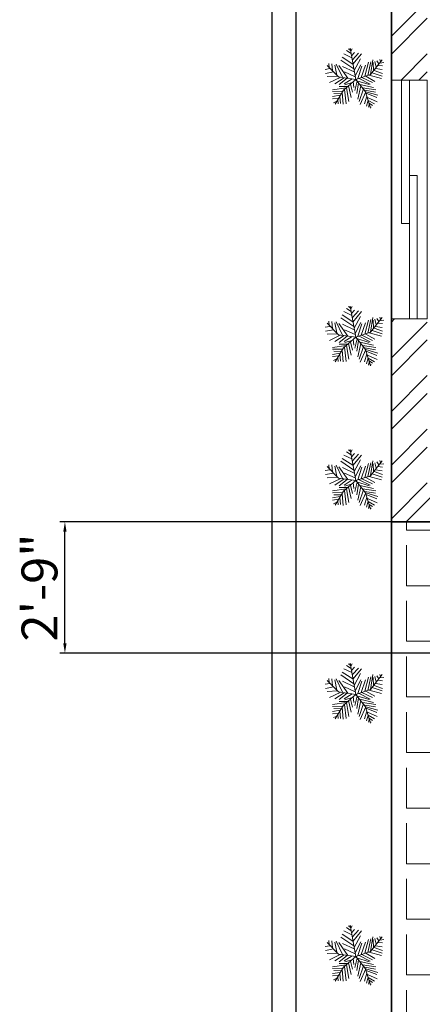
# Model space of a CAD drawing. Units: inches. Extents: x 889 to 1572, y 7262 to 8387.
# Tile 1 of 8: x 923 to 1024, y 7495 to 7742. Entities that reach past the tile are written whole.
import ezdxf

# ---------------------------------------------------------------- set-up
doc = ezdxf.new("R2010")
doc.units = ezdxf.units.IN
for name, color, linetype, lineweight in [('A-ANNO-DIMS', 2, 'Continuous', 18), ('A-WALL', 7, 'Continuous', 35), ('A-WALL-PATT', 252, 'Continuous', 13), ('C-SITE', 7, 'Continuous', 30), ('L-PLNT', 94, 'Continuous', 13), ('L-PVMT-PATT', 252, 'Continuous', 13)]:
    doc.layers.add(name, color=color, linetype=linetype, lineweight=lineweight)
doc.layers.add('A-GLAZ', color=244, linetype='Continuous', lineweight=18, true_color=0x991b1e)
doc.styles.get("Standard").update_dxf_attribs({"font": 'arial.ttf'})
doc.dimstyles.new('ISO-25', dxfattribs={"dimtxt": 9, "dimasz": 2.5, "dimexe": 1.25, "dimexo": 0.625, "dimtad": 1, "dimlunit": 3, "dimtxsty": 'Standard', "dimcen": 2.5, "dimadec": 0, "dimazin": 0, "dimtfac": 1, "dimtmove": 0, "dimatfit": 3, "dimfxl": 1, "dimarcsym": 0})

# ---------------------------------------------------------------- blocks, each defined once
blk = doc.blocks.new('*U15')
for p, q in [((-10.18600000000015, 53.63999999999987), (-13.08399999999983, 55.96199999999976)), ((0, 0), (-10.5, 57)), ((-9.098999999999705, 51.7819999999997), (-6.563000000000101, 55.96199999999976)), ((-5.114000000000032, 28.09699999999975), (-24.67599999999993, 40.63599999999996)), ((-7.28800000000001, 39.70699999999965), (-21.77800000000025, 46.67299999999977)), ((-8.736999999999625, 47.13799999999969), (-17.06899999999996, 52.71100000000001)), ((-7.65000000000009, 43.42299999999977), (-2.577999999999974, 49.45999999999981)), ((-5.838999999999941, 35.99199999999973), (4.666999999999916, 48.06699999999977)), ((-5.114000000000032, 27.63199999999983), (10.46300000000019, 46.67299999999977)), ((-2.940999999999803, 16.48599999999987), (8.652000000000044, 37.84999999999991)), ((27, 9), (48, 36)), ((27.12699999999995, 9.05600000000004), (31.11200000000008, 35.99199999999973)), ((44.15300000000025, 36.45599999999991), (45.23900000000003, 32.74099999999999)), ((-47.49800000000004, 19.73699999999962), (-55.83000000000038, 18.34399999999982)), ((-31.5, 4.5), (-52.5, 25.5)), ((-48.58500000000003, 21.13099999999986), (-49.30899999999974, 29.02600000000007)), ((-43.51299999999992, 28.56099999999992), (-42.42699999999968, 15.55799999999976)), ((-38.44199999999955, 26.23899999999981), (-34.81899999999996, 7.662999999999783)), ((-35.54399999999987, 28.09699999999975), (-24.31399999999985, 3.946999999999661)), ((-14.5329999999999, 2.089999999999918), (-30.83399999999983, 25.30999999999995)), ((-3.665000000000418, 19.27299999999968), (-27.57400000000007, 35.52699999999982)), ((-24.31399999999985, 23.91699999999969), (-2.940999999999803, 13.69999999999982)), ((-1.128999999999905, 6.733999999999923), (9.014000000000124, 26.70399999999995)), ((3.942000000000007, 1.625), (11.1869999999999, 24.38099999999986)), ((10.10100000000011, 3.482999999999719), (17.70800000000008, 26.23899999999981)), ((16.25900000000001, 5.804999999999836), (23.14199999999983, 31.34799999999973)), ((22.05499999999984, 7.197999999999865), (27.48900000000003, 32.27699999999982)), ((31.83600000000024, 30.88299999999981), (32.56100000000015, 16.48599999999987)), ((35.09600000000001, 32.74099999999999), (37.26999999999998, 22.52399999999989)), ((36.18300000000045, 19.73699999999962), (48.13699999999972, 17.87999999999988)), ((38.71900000000005, 34.13399999999979), (41.97899999999981, 28.56099999999992)), ((40.52999999999975, 25.77499999999986), (48.86200000000008, 24.846)), ((43.79100000000017, 29.95399999999995), (51.03600000000006, 30.88299999999981)), ((-40.61500000000023, 13.69999999999982), (-55.10500000000002, 10.91299999999978)), ((-33.37000000000035, 6.268999999999778), (-52.20699999999988, 5.339999999999918)), ((-28.29899999999998, 3.482999999999719), (-47.86000000000012, -5.805000000000063)), ((-21.41600000000017, 3.017999999999801), (-38.07899999999973, -8.128000000000384)), ((0, 0), (-31.5, 4.5)), ((-15.98199999999951, 2.089999999999918), (-30.11000000000013, -9.521000000000186)), ((0, 0), (-22.5, -19.5)), ((-6.563000000000101, 1.161000000000058), (-21.41600000000017, -8.128000000000384)), ((-20.69099999999981, 13.69999999999982), (-1.128999999999905, 4.875999999999976)), ((0, 0), (27, 9)), ((0, 0), (18, -22.5)), ((6.478000000000065, 1.625), (26.03999999999996, -8.592000000000326)), ((11.1869999999999, 3.482999999999719), (30.74900000000025, -5.805000000000063)), ((18.06999999999971, 5.804999999999836), (35.09600000000001, -3.483000000000174)), ((24.22899999999982, 7.662999999999783), (46.6880000000001, 1.625)), ((29.66199999999981, 12.30699999999979), (48.13699999999972, 6.268999999999778)), ((33.28499999999986, 16.48599999999987), (48.86200000000008, 10.91299999999978)), ((-17.43100000000004, -15.09400000000005), (-42.78899999999976, -18.80899999999997)), ((-15.2569999999996, -12.77200000000016), (-30.11000000000013, -12.77200000000016)), ((-6.563000000000101, -5.805000000000063), (-19.96699999999964, -9.985000000000127)), ((-17.06899999999996, -15.09400000000005), (-12.721, -40.17200000000025)), ((-13.44599999999991, -11.37800000000038), (-8.736999999999625, -32.74100000000021)), ((-9.460999999999785, -8.592000000000326), (-6.201000000000021, -23.4530000000002)), ((-4.751999999999952, -3.483000000000174), (-3.665000000000418, -14.62900000000013)), ((2.493000000000392, -3.019000000000005), (-1.490999999999985, -20.20200000000023)), ((1.769000000000232, -2.555000000000063), (24.22899999999982, -9.521000000000186)), ((5.028999999999996, -6.270000000000209), (2.131000000000312, -25.77500000000009)), ((9.014000000000124, -11.37800000000038), (3.579999999999927, -35.99200000000019)), ((14.08499999999958, -16.95100000000025), (6.478000000000065, -40.17200000000025)), ((7.564999999999599, -9.056000000000267), (32.19800000000032, -14.62900000000013)), ((12.27399999999988, -15.09400000000005), (36.9069999999997, -18.80899999999997)), ((-28.29899999999998, -29.02600000000007), (-42.78899999999976, -31.34800000000018)), ((-24.31399999999985, -21.59600000000023), (-42.42699999999968, -22.06000000000017)), ((-30.83399999999983, -34.13499999999999), (-42.42699999999968, -35.52800000000025)), ((-26.8489999999997, -26.24000000000001), (-40.25300000000015, -25.77500000000009)), ((-22.5, -19.5), (-37.5, -45)), ((-29.02300000000014, -30.88400000000002), (-27.93600000000015, -43.88700000000016)), ((-25.03800000000001, -23.91800000000035), (-22.86500000000024, -45.28100000000017)), ((-20.69099999999981, -18.34500000000003), (-17.79300000000012, -44.35200000000032)), ((18.06999999999971, -22.52400000000012), (8.289000000000215, -45.74500000000012)), ((20.24400000000014, -30.4190000000001), (15.89699999999993, -44.81600000000026)), ((16.25900000000001, -19.73800000000028), (36.18300000000045, -22.98900000000003)), ((18, -22.5), (27, -52.5)), ((18.43300000000045, -22.52400000000012), (40.52999999999975, -29.02600000000007)), ((19.1569999999997, -25.31100000000015), (38.71900000000005, -33.20600000000013)), ((21.33100000000013, -32.74100000000021), (39.08100000000013, -40.63600000000019)), ((-34.45699999999988, -39.70800000000031), (-40.97800000000006, -42.49400000000014)), ((-32.64600000000019, -36.92100000000005), (-31.92099999999982, -44.35200000000032)), ((22.77999999999975, -37.85000000000014), (19.51900000000023, -48.53200000000015)), ((22.77999999999975, -38.31400000000008), (34.37199999999985, -44.81600000000026)), ((24.59100000000035, -45.74500000000012), (23.14199999999983, -50.85400000000004)), ((24.59100000000035, -43.42300000000022), (30.74900000000025, -47.60300000000029)), ((26.76400000000012, -49.92500000000018), (28.21300000000019, -50.85400000000004))]:
    blk.add_line(p, q)
blk = doc.blocks.new('GLAZ-SLIDER-60IN')
for p, q in [((-0.0003915866479929, 60.00023087260706), (-0.0003915866479929, 24.00023087260706)), ((1.999608413352007, 60.00023087260706), (1.999608413352007, 0.0002308726070623)), ((1.999608413352007, 36.00023087260706), (3.999608413352007, 36.00023087260706)), ((3.999608413352007, 36.00023087260706), (3.999608413352007, 0.0002308726070623)), ((1.999608413352007, 24.00023087260706), (-0.0003915866479929, 24.00023087260706))]:
    blk.add_line(p, q)
blk = doc.blocks.new('*D69')
at = {"layer": 'A-ANNO-DIMS', "color": 0, "lineweight": -2, "transparency": 16777216}
for p, q in [((1016.048608, 7615.106231), (1016.048608, 7262.354215000001)), ((1436.048608, 7582.106231), (1436.048608, 7262.354215000001)), ((1018.548608, 7263.604215), (1433.548608, 7263.604215))]:
    blk.add_line(p, q, dxfattribs=at)
at = {"layer": 'A-ANNO-DIMS', "color": 0, "transparency": 16777216}
for points in [[(1018.548608, 7264.020881666667), (1018.548608, 7263.187548333333), (1016.048608, 7263.604215)], [(1433.548608, 7264.020881666667), (1433.548608, 7263.187548333333), (1436.048608, 7263.604215)]]:
    blk.add_solid(points, dxfattribs=at)
at = {"layer": 'Defpoints', "color": 0, "transparency": 16777216}
for p in [(1016.048608, 7615.731230999999), (1436.048608, 7582.731231), (1436.048608, 7263.604215)]:
    blk.add_point(p, dxfattribs=at)
at = {"layer": 'A-ANNO-DIMS', "color": 0, "transparency": 16777216, "insert": (1226.048608, 7268.827441466576), "char_height": 9, "attachment_point": 5}
blk.add_mtext('35\'-0"', dxfattribs=at)
blk = doc.blocks.new('*D72')
at = {"layer": 'A-ANNO-DIMS', "color": 0, "lineweight": -2, "transparency": 16777216}
for p, q in [((1204.423608, 7615.731231000004), (932.7986080000009, 7615.731231000004)), ((934.0486080000009, 7585.231231000003), (934.0486080000009, 7613.231231000003)), ((1204.423608, 7582.731231000003), (932.7986080000009, 7582.731231000003))]:
    blk.add_line(p, q, dxfattribs=at)
at = {"layer": 'A-ANNO-DIMS', "color": 0, "transparency": 16777216}
for points in [[(933.6319413333342, 7613.231231000003), (934.4652746666675, 7613.231231000003), (934.0486080000009, 7615.731231000004)], [(933.6319413333342, 7585.231231000003), (934.4652746666675, 7585.231231000003), (934.0486080000009, 7582.731231000003)]]:
    blk.add_solid(points, dxfattribs=at)
at = {"layer": 'Defpoints', "color": 0, "transparency": 16777216}
for p in [(934.0486080000009, 7615.731231000004), (1205.048608, 7615.731231000004), (1205.048608, 7582.731231000003)]:
    blk.add_point(p, dxfattribs=at)
at = {"layer": 'A-ANNO-DIMS', "color": 0, "transparency": 16777216, "insert": (928.8284511105074, 7599.231231000001), "char_height": 9, "attachment_point": 5, "rotation": 90}
blk.add_mtext('2\'-9"', dxfattribs=at)

msp = doc.modelspace()

# ---------------------------------------------------------------- hatches: boundary and pattern name
at = {"layer": 'A-WALL-PATT'}
h = msp.add_hatch(dxfattribs=at)
h.set_pattern_fill('ANSI32', color=256)
h.set_pattern_definition([(45, (0, 0), (-6.735192090801866, 6.735192090801866), []), (45, (4.49013, 0), (-6.735192090801866, 6.735192090801866), [])])
h.paths.add_polyline_path([(1166.048608413352, 7624.731230872604), (1163.048608413352, 7624.731230872604), (1163.048608413352, 7774.731230872602), (1154.048608413352, 7774.731230872602), (1154.048608413352, 7768.731230872603), (1157.048608413352, 7768.731230872603), (1157.048608413352, 7624.731230872604), (1106.048608413347, 7624.731230872605), (1106.048608413347, 7615.731230872604), (1166.048608413352, 7615.731230872604), (1166.048608413352, 7618.431230872605)])
h.paths.add_polyline_path([(1025.048608413352, 7666.731230872606), (1016.048608413352, 7666.731230872606), (1016.048608413352, 7615.731230872608), (1076.048608413347, 7615.731230872606), (1076.048608413347, 7624.731230872605), (1025.048608413352, 7624.731230872606)])
h.paths.add_polyline_path([(1025.048608413352, 7768.731230872607), (1118.048608413352, 7768.731230872605), (1118.048608413352, 7774.731230872603), (1025.048608413352, 7774.731230872607), (1025.048608413352, 7897.731230872607), (1115.048608413351, 7897.731230872603), (1115.048608413351, 7906.731230872605), (1109.048608413352, 7906.731230872605), (1109.048608413352, 7903.731230872605), (1025.048608413352, 7903.731230872607), (1025.048608413352, 7923.231230872606), (1016.048608413352, 7923.231230872606), (1016.048608413352, 7726.731230872608), (1025.048608413352, 7726.731230872608)])
h.paths.add_polyline_path([(1436.048608413352, 7897.731230872607), (1427.048608413351, 7897.731230872607), (1427.048608413351, 7883.37377559743), (1436.048608413352, 7883.37377559743)])
h.paths.add_polyline_path([(1436.048608413352, 7853.373775597429), (1427.048608413351, 7853.373775597429), (1427.048608413351, 7843.731230872608), (1415.048608413352, 7843.731230872608), (1415.048608413352, 7837.731230872607), (1427.048608413351, 7837.731230872607), (1427.048608413351, 7831.731230872607), (1436.048608413352, 7831.731230872607)])
h.paths.add_polyline_path([(1436.048608413352, 8010.183478752281), (1427.048608413351, 8010.183478752281), (1427.048608413351, 7970.456226002662), (1370.048608413352, 7970.456226002662), (1370.048608413352, 7963.731230872607), (1427.048608413351, 7963.731230872608), (1427.048608413351, 7957.731230872607), (1436.048608413352, 7957.731230872607)])
h.paths.add_polyline_path([(1436.048608413352, 7747.731230872607), (1427.048608413352, 7747.731230872607), (1427.048608413352, 7741.731230872608), (1344.721387503392, 7741.731230872608), (1344.721387503392, 7735.731230872609), (1349.048608413352, 7735.731230872609), (1349.048608413352, 7672.731230872607), (1355.048608413352, 7672.731230872606), (1355.048608413352, 7735.731230872609), (1427.048608413352, 7735.731230872608), (1427.048608413352, 7721.931475650177), (1436.048608413352, 7721.931475650177)])
h.paths.add_polyline_path([(1436.048608413352, 7700.931475650178), (1427.048608413352, 7700.931475650178), (1427.048608413352, 7591.731230872608), (1355.048608413352, 7591.731230872608), (1355.048608413352, 7642.731230872605), (1349.048608413352, 7642.731230872607), (1349.048608413352, 7591.731230872608), (1310.048608413352, 7591.731230872608), (1310.048608413352, 7582.731230872609), (1436.048608413352, 7582.731230872608)])
h.paths.add_polyline_path([(1392.41988820942, 8272.731230872607), (1331.048608413352, 8272.731230872607), (1331.048608413352, 8263.731230872607), (1349.048608413352, 8263.731230872607), (1349.048608413352, 8224.731230872603), (1355.048608413352, 8224.731230872607), (1355.048608413352, 8263.731230872607), (1392.41988820942, 8263.731230872607)])
h.paths.add_polyline_path([(1271.048608413352, 8272.731230872607), (1196.736043973615, 8272.731230872607), (1196.736043973615, 8263.731230872607), (1247.048608413352, 8263.731230872607), (1247.048608413352, 8203.731230872605), (1244.048608413352, 8203.731230872605), (1244.048608413352, 8197.731230872605), (1247.048608413352, 8197.731230872605), (1247.048608413353, 8161.731230872605), (1253.048608413352, 8161.731230872605), (1253.048608413352, 8185.731230872605), (1295.048608413353, 8185.731230872603), (1295.048608413353, 8191.731230872607), (1253.048608413352, 8191.731230872605), (1253.048608413352, 8263.731230872607), (1271.048608413352, 8263.731230872607)])
h.paths.add_polyline_path([(1175.736043973615, 8272.731230872607), (1102.037311183427, 8272.731230872607), (1102.037311183427, 8263.731230872607), (1157.048608413352, 8263.731230872607), (1157.048608413352, 8158.731230872607), (1163.048608413352, 8158.731230872607), (1163.048608413352, 8197.731230872605), (1214.048608413352, 8197.731230872605), (1214.048608413352, 8203.731230872605), (1163.048608413352, 8203.731230872605), (1163.048608413352, 8263.731230872607), (1175.736043973615, 8263.731230872607)])
h.paths.add_polyline_path([(1072.037311183427, 8272.731230872607), (1016.048608413352, 8272.731230872607), (1016.048608413352, 8221.731230872607), (1025.048608413352, 8221.731230872607), (1025.048608413352, 8263.731230872607), (1072.037311183427, 8263.731230872607)])
h.paths.add_polyline_path([(1163.048608413352, 8122.731230872608), (1157.048608413352, 8122.731230872608), (1157.048608413352, 8119.731230872607), (1025.048608413352, 8119.731230872607), (1025.048608413352, 8161.731230872607), (1016.048608413352, 8161.731230872607), (1016.048608413352, 8071.731230872606), (1025.048608413352, 8071.731230872606), (1025.048608413352, 8113.731230872607), (1157.048608413352, 8113.731230872607), (1157.048608413352, 8110.731230872607), (1163.048608413352, 8110.731230872607)])
h.paths.add_polyline_path([(1025.048608413352, 8011.731230872607), (1016.048608413352, 8011.731230872607), (1016.048608413352, 7944.231230872607), (1025.048608413352, 7944.231230872607), (1025.048608413352, 7963.731230872607), (1109.048608413352, 7963.731230872605), (1109.048608413352, 7936.731230872606), (1115.048608413351, 7936.731230872606), (1115.048608413351, 7963.731230872605), (1163.048608413352, 7963.731230872607), (1163.048608413352, 8074.731230872606), (1157.048608413352, 8074.731230872606), (1157.048608413352, 7969.731230872607), (1025.048608413352, 7969.731230872607)])
h.paths.add_polyline_path([(1314.721387503392, 7741.731230872608), (1307.048608413352, 7741.731230872608), (1307.048608413352, 7837.731230872609), (1319.048608413352, 7837.731230872609), (1319.048608413352, 7843.731230872608), (1307.048608413352, 7843.731230872608), (1307.048608413352, 7963.731230872608), (1310.048608413352, 7963.731230872607), (1310.048608413352, 7970.456226002662), (1301.048608413352, 7970.456226002662), (1301.048608413352, 7837.731230872607), (1301.048608413352, 7741.731230872608), (1250.048608413352, 7741.731230872608), (1250.048608413352, 7735.731230872609), (1314.721387503392, 7735.731230872609)])
h.paths.add_polyline_path([(1211.048608413352, 7735.731230872609), (1214.048608413352, 7735.731230872609), (1214.048608413352, 7741.731230872608), (1205.048608413352, 7741.731230872608), (1205.048608413352, 7624.731230872601), (1202.048608413352, 7624.731230872602), (1202.048608413352, 7615.731230872603), (1205.048608413352, 7615.731230872604), (1205.048608413352, 7582.731230872609), (1250.048608413353, 7582.731230872609), (1250.048608413353, 7591.73123087261), (1211.048608413352, 7591.731230872611)])
h.paths.add_polyline_path([(1436.048608413352, 8260.718366180157), (1427.048608413352, 8260.718366180157), (1427.048608413351, 8191.731230872607), (1355.048608413352, 8191.731230872607), (1355.048608413352, 8194.731230872607), (1349.048608413352, 8194.731230872603), (1349.048608413352, 8191.731230872607), (1343.048608413353, 8191.731230872607), (1343.048608413353, 8185.731230872608), (1427.048608413352, 8185.731230872608), (1427.048608413351, 8070.183478752282), (1436.048608413352, 8070.183478752282)])
at = {"layer": 'L-PVMT-PATT'}
h = msp.add_hatch(dxfattribs=at)
h.set_pattern_fill('ANGLE', color=256, scale=2)
h.set_pattern_definition([(0, (0, 0), (0, 13.97), [10.16, -3.81]), (90, (0, 0), (-13.97, 9e-16), [10.16, -3.81])])
h.paths.add_polyline_path([(1205.048608413351, 7555.446171834415), (1204.522810014118, 7555.264684699134), (1205.048608413351, 7555.910703335377), (1205.048608413352, 7557.193763035785), (1204.375295363129, 7557.060960744141), (1205.048608413352, 7557.600559978721), (1205.048608413352, 7559.617877481), (1204.375295363129, 7559.330134346581), (1204.006412068125, 7559.046511813157), (1204.08026606115, 7559.708297724476), (1205.048608413352, 7561.087614386948), (1205.048608413352, 7561.676628270497), (1205.03901462505, 7561.693848793495), (1204.227780712139, 7562.166553015865), (1205.048608413352, 7562.166553015865), (1205.048608413352, 7565.277573844389), (1205.03901462505, 7565.286594218571), (1205.048608413352, 7565.286594218571), (1205.048608413352, 7578.731230872603), (1159.234402724352, 7578.731230872605), (1159.234402724352, 7578.363210835082, -0.1960004452144572), (1159.622195581334, 7577.411949376209, -1.441243748687975), (1157.234402724352, 7578.304265881411), (1157.234402724352, 7615.731230872604), (1016.048608413352, 7615.731230872608), (1016.048608413352, 7399.731230872607), (1022.048608413351, 7399.731230872605), (1205.048608413347, 7399.731230872603), (1205.048608413347, 7402.731230872603)])
edge = h.paths.add_edge_path(flags=16)
edge.add_ellipse((-9486.215667076898, 7539.371191098851), major_axis=(10593.02630634627, 3.017206e-10), ratio=0.8423038695454096, start_angle=-0.38386677879407216, end_angle=0.09022908859270728, ccw=False)
edge.add_ellipse((1106.81063926937, 7467.155380808408), major_axis=(1.479846074908209, 2.4527e-12), ratio=0.8423038695436039, start_angle=-9.487166607868858e-11, end_angle=89.99999999990501, ccw=False)
edge.add_line((1108.290485344278, 7467.155380808408), (1108.290485344278, 7442.952241603949))
edge.add_ellipse((1106.81063926937, 7442.952241603949), major_axis=(-1.479846074908209, 2.4527e-12), ratio=0.8423038695436041, start_angle=90.00000000009499, end_angle=180.0000000000949, ccw=False)
edge.add_line((1106.81063926937, 7441.705761528725), (1106.176028993391, 7441.705761528725))
edge.add_ellipse((-9486.215667076898, 7539.371191098851), major_axis=(10593.02630634627, 3.017206e-10), ratio=0.8423038695454096, start_angle=-0.6186431963208179, end_angle=-0.5282714718196075, ccw=False)
edge.add_ellipse((1105.240175582287, 7423.225144549206), major_axis=(2.219769112362271, 3.512e-12), ratio=0.8423038695437586, start_angle=-0.6282372162759771, end_angle=68.464756600913, ccw=False)
edge.add_ellipse((-9486.955590114589, 7539.371191096425), major_axis=(-10595.31303979869, 5.7334850558e-06), ratio=0.8423038635969176, start_angle=179.3534459339559, end_angle=179.3717628147891, ccw=False)
edge.add_ellipse((1102.160695079015, 7419.873259495446), major_axis=(-5.246425615115091, 6.131e-13), ratio=0.8423038695439657, start_angle=90.00000000006861, end_angle=179.3534459029308, ccw=False)
edge.add_line((1102.16069507902, 7415.45417489856), (1036.643322523875, 7415.454174898562))
edge.add_ellipse((1036.643322523886, 7419.87325949545), major_axis=(5.246425615118246, 3.3658e-12), ratio=0.8423038695439792, start_angle=180.6465540970289, end_angle=269.9999999998247, ccw=False)
edge.add_ellipse((11625.75960776125, 7539.371191101991), major_axis=(-10595.31303986147, 2.5904085676e-06), ratio=0.8423038722500887, start_angle=0.6282372302511021, end_angle=0.6465541110841855, ccw=False)
edge.add_ellipse((1033.56384202061, 7423.225144549211), major_axis=(2.219769112362928, 1.9515e-12), ratio=0.8423038695441785, start_angle=111.5352435039708, end_angle=180.6282372161348, ccw=False)
edge.add_ellipse((11625.0196847094, 7539.371191099013), major_axis=(-10593.02630637587, 5.863276e-10), ratio=0.8423038695454017, start_angle=0.528271471820517, end_angle=0.646554097064211, ccw=False)
edge.add_line((1032.627988609511, 7441.705761528725), (1031.993378333528, 7441.705761528725))
edge.add_ellipse((1031.993378333528, 7442.952241603949), major_axis=(1.479846074908209, 2.4527e-12), ratio=0.8423038695436039, start_angle=179.999999999905, end_angle=269.999999999905, ccw=False)
edge.add_line((1030.51353225862, 7442.952241603949), (1030.51353225862, 7467.155380808408))
edge.add_ellipse((1031.993378333528, 7467.155380808408), major_axis=(-1.479846074908209, 2.4527e-12), ratio=0.8423038695436041, start_angle=-89.99999999990501, end_angle=9.498535291641019e-11, ccw=False)
edge.add_ellipse((11625.0196847094, 7539.371191099013), major_axis=(-10593.02630637587, 5.863276e-10), ratio=0.8423038695454017, start_angle=-0.0902290885899788, end_angle=0.38386677879549325, ccw=False)
edge.add_ellipse((1031.993378333528, 7557.299497249569), major_axis=(-1.479846074907982, 9.504e-13), ratio=0.8423038695443477, start_angle=3.6777692002942786e-11, end_angle=90.00000000003672, ccw=False)
edge.add_line((1030.51353225862, 7557.299497249569), (1030.51353225862, 7581.502636454029))
edge.add_ellipse((1031.993378333528, 7581.502636454029), major_axis=(-1.479846074907982, 2.1793e-12), ratio=0.8423038695437334, start_angle=-89.99999999991559, end_angle=8.44124770082999e-11, ccw=False)
edge.add_line((1031.993378333528, 7582.749116529253), (1032.569706643912, 7582.749116529253))
edge.add_ellipse((1560.265112694065, 7562.662031955335), major_axis=(528.2339998381949, 5.3105e-12), ratio=0.8423038695440039, start_angle=176.3495724143003, end_angle=177.8200496863542, ccw=False)
edge.add_ellipse((1096.926435685115, 7337.82316262669), major_axis=(-313.3077612789123, 2.032944e-09), ratio=0.84230386954869, start_angle=-77.87403444734417, end_angle=-76.21947101013029, ccw=False)
edge.add_ellipse((1096.926435685109, 7344.678164312899), major_axis=(-305.3028914625973, 2.877231e-10), ratio=0.842303869544824, start_angle=-79.79046100280272, end_angle=-77.55537270650188, ccw=False)
edge.add_ellipse((1017.005159108514, 7808.347848963542), major_axis=(250.9602162202823, 3.689106e-10), ratio=0.8423038695427255, start_angle=-80.7434339928827, end_angle=-77.44506735594696)
edge.add_line((1063.273718708008, 7600.586721862112), (1069.402008801449, 7603.975488617634))
edge.add_line((1069.402008801449, 7603.975488617634), (1075.53029889489, 7600.586721862112))
edge.add_ellipse((1121.798858494384, 7808.347848963542), major_axis=(-250.9602162202835, 3.684091e-10), ratio=0.8423038695427219, start_angle=77.44506735594675, end_angle=80.74343399288247)
edge.add_ellipse((1041.877581917783, 7344.678164312894), major_axis=(305.3028914626093, 3.003322e-10), ratio=0.842303869544806, start_angle=77.55537270649842, end_angle=79.79046100279919, ccw=False)
edge.add_ellipse((1041.877581917783, 7337.82316262669), major_axis=(313.3077612789065, 2.0431705e-09), ratio=0.8423038695487045, start_angle=76.21947101012842, end_angle=77.87403444734218, ccw=False)
edge.add_ellipse((578.5389049088338, 7562.662031955335), major_axis=(-528.2339998381949, 1.51629e-11), ratio=0.8423038695441082, start_angle=182.1799503136469, end_angle=183.6504275857008, ccw=False)
edge.add_line((1106.234310958986, 7582.749116529253), (1106.81063926937, 7582.749116529253))
edge.add_ellipse((1106.81063926937, 7581.502636454029), major_axis=(1.479846074908209, 2.4524e-12), ratio=0.8423038695436039, start_angle=-9.487166607868858e-11, end_angle=89.99999999989461, ccw=False)
edge.add_line((1108.290485344278, 7581.502636454029), (1108.290485344278, 7557.299497249569))
edge.add_ellipse((1106.81063926937, 7557.299497249569), major_axis=(1.479846074908209, 6.78e-13), ratio=0.8423038695442183, start_angle=269.99999999997374, end_angle=359.9999999999738, ccw=False)
edge = h.paths.add_edge_path(flags=0)
edge.add_ellipse((-9486.215667106499, 7539.371191098978), major_axis=(10591.54646030096, 1.2635629e-09), ratio=0.8423038695462665, start_angle=-0.3777641939166756, end_angle=-0.055594313506105664, ccw=False)
edge.add_line((1105.006318572806, 7469.539827495825), (1101.179586793223, 7484.564921120725))
edge.add_ellipse((-2596.951337496201, 7508.064385441264), major_axis=(3698.23615920963, 2.129104e-10), ratio=0.8423038695460041, start_angle=-0.3640763488936447, end_angle=0.1208973690293594)
edge.add_line((1101.273217526047, 7515.867862174639), (1105.323765593278, 7529.094176745418))
edge = h.paths.add_edge_path(flags=0)
edge.add_line((1100.938139695363, 7533.822901558612), (1098.75325771553, 7517.447032490746))
edge.add_ellipse((1072.201451338588, 7454.257822231051), major_axis=(-79.57966406428197, 3.36667e-11), ratio=0.8423038695436982, start_angle=247.2080851224342, end_angle=265.1299304028885)
edge.add_line((1077.898048720122, 7521.116122104183), (1060.905968882777, 7521.116122104183))
edge.add_ellipse((1066.602566264312, 7454.257822231035), major_axis=(79.57966406429925, 3.47446e-11), ratio=0.842303869543722, start_angle=94.87006959711071, end_angle=112.7919148775615)
edge.add_line((1040.050759887368, 7517.447032490746), (1037.865877907535, 7533.822901558612))
edge.add_ellipse((1064.014567125969, 7468.562006392521), major_axis=(81.77258453066123, 3.0009e-12), ratio=0.8423038695439617, start_angle=94.27742096305201, end_angle=111.8349537967062, ccw=False)
edge.add_line((1058.873140668548, 7537.30309200137), (1079.930876934351, 7537.30309200137))
edge.add_ellipse((1074.789450476928, 7468.562006392524), major_axis=(81.77258453065926, 1.3305e-12), ratio=0.8423038695439597, start_angle=68.16504620328942, end_angle=85.7225790369435, ccw=False)
edge = h.paths.add_edge_path(flags=0)
edge.add_ellipse((1082.739732964455, 7553.062906659881), major_axis=(0.3566085810348156, 6.340077547122254), ratio=0.6038335755719637, start_angle=106.3425919542708, end_angle=270.9979857249622, ccw=False)
edge.add_line((1078.907842185069, 7552.169556028257), (1078.907842185069, 7574.080393839259))
edge.add_ellipse((1022.738983135553, 7574.080393839259), major_axis=(-56.16885904951628, 2.3357e-12), ratio=0.8423038695439936, start_angle=180.0000000000023, end_angle=209.4385695979816)
edge.add_ellipse((1116.065034467345, 7574.080393839259), major_axis=(56.16885904951618, 2.2359e-12), ratio=0.8423038695439938, start_angle=150.5614304020184, end_angle=179.9999999999977)
edge.add_line((1059.896175417829, 7574.08039383926), (1059.896175417829, 7552.169556028257))
edge.add_ellipse((1056.064284638443, 7553.062906659881), major_axis=(-0.3566085810390883, 6.340077547122437), ratio=0.6038335755718836, start_angle=89.00201427499962, end_angle=253.6574080456915, ccw=False)
edge.add_line((1052.232393859057, 7552.914272145777), (1052.232393859057, 7567.724446781444))
edge.add_line((1052.232393859057, 7567.724446781444), (1057.981948927734, 7571.730267706323))
edge.add_line((1057.981948927734, 7571.730267706323), (1059.896175417829, 7571.730267706323))
edge.add_line((1059.896175417829, 7571.730267706323), (1059.896175417829, 7574.08039383926))
edge.add_ellipse((1116.065034467345, 7574.080393839259), major_axis=(56.16885904951618, 2.2359e-12), ratio=0.8423038695439938, start_angle=150.5614304020184, end_angle=179.9999999999977, ccw=False)
edge.add_ellipse((1022.738983135553, 7574.080393839259), major_axis=(-56.16885904951628, 2.3357e-12), ratio=0.8423038695439936, start_angle=180.0000000000024, end_angle=209.4385695979817, ccw=False)
edge.add_line((1078.907842185069, 7574.080393839259), (1078.907842185069, 7571.730267706323))
edge.add_line((1078.907842185069, 7571.730267706323), (1080.822068675164, 7571.730267706323))
edge.add_line((1080.822068675164, 7571.730267706323), (1086.571623743841, 7567.724446781444))
edge.add_line((1086.571623743841, 7567.724446781444), (1086.571623743841, 7552.914272145774))
edge = h.paths.add_edge_path(flags=0)
edge.add_line((1098.75325771553, 7465.430300647797), (1098.75325771553, 7446.606616602368))
edge.add_ellipse((1069.402008801449, 7567.947422636645), major_axis=(-147.017923889832, 1.396e-13), ratio=0.8423038695439693, start_angle=76.4018653097695, end_angle=103.59813469023061, ccw=False)
edge.add_line((1040.050759887368, 7446.606616602368), (1040.050759887368, 7465.430300647797))
edge.add_ellipse((1069.402008801449, 7586.771106682075), major_axis=(-147.017923889832, 1.396e-13), ratio=0.8423038695439693, start_angle=76.4018653097695, end_angle=103.5981346902306)
edge = h.paths.add_edge_path(flags=0)
edge.add_ellipse((1095.793565565714, 7436.844830295861), major_axis=(-2.959692149816191, 1.9947e-12), ratio=0.842303869543976, start_angle=180.0000000000387, end_angle=270.0000000000386, ccw=False)
edge.add_line((1098.75325771553, 7436.844830295861), (1098.75325771553, 7417.380299344997))
edge.add_line((1098.75325771553, 7417.380299344997), (1040.050759887368, 7417.380299344998))
edge.add_line((1040.050759887368, 7417.380299344998), (1040.050759887368, 7436.844830295861))
edge.add_ellipse((1043.010452037184, 7436.844830295861), major_axis=(2.959692149816192, 1.9928e-12), ratio=0.8423038695439758, start_angle=89.9999999999614, end_angle=179.9999999999614, ccw=False)
edge.add_line((1043.010452037184, 7439.337790446311), (1095.793565565714, 7439.337790446311))
edge = h.paths.add_edge_path(flags=0)
edge.add_ellipse((4735.755355099098, 7508.064385441248), major_axis=(-3698.236159209629, 1.078002e-10), ratio=0.8423038695486287, start_angle=-0.1208973690313006, end_angle=0.3640763488917358)
edge.add_line((1037.624430809674, 7484.564921120725), (1033.797699030094, 7469.539827495835))
edge.add_ellipse((11625.01968470938, 7539.371191098929), major_axis=(10591.54646030094, 2.5735131e-09), ratio=0.8423038695346576, start_angle=180.0555943134852, end_angle=180.3777641938957, ccw=False)
edge.add_line((1033.480252009621, 7529.094176745418), (1037.530800076852, 7515.867862174644))
h.paths.add_polyline_path([(1109.981626785864, 7408.740466663437), (1190.985719555305, 7408.740466663437), (1190.985719555305, 7438.592217459254), (1109.981626785864, 7438.592217459254)], flags=24)

# ---------------------------------------------------------------- linework, layer by layer
at = {"layer": 'A-GLAZ'}
msp.add_lwpolyline([(1016.048608413352, 7726.731230872608), (1025.048608413352, 7726.731230872608), (1025.048608413352, 7666.731230872606), (1016.048608413352, 7666.731230872606)], close=True, dxfattribs=at)
at = {"layer": 'A-WALL'}
for p, q in [((1016.048608413352, 8272.731230872607), (1016.048608413352, 7393.731230872607)), ((1016.048608413352, 7615.731230872608), (1166.048608413352, 7615.731230872604))]:
    msp.add_line(p, q, dxfattribs=at)
at = {"layer": 'C-SITE'}
for p, q in [((986.0486084133516, 8272.731230872607), (986.0486084133516, 7393.731230872607)), ((992.0486084133518, 8272.731230872607), (992.0486084133518, 7405.731230872598))]:
    msp.add_line(p, q, dxfattribs=at)

# ---------------------------------------------------------------- block references
at = {"layer": 'A-GLAZ', "rotation": 180}
msp.add_blockref('GLAZ-SLIDER-60IN', (1022.548216826703, 7726.731461745216), dxfattribs=at)
at = {"layer": 'L-PLNT', "xscale": 0.137481440781912, "yscale": 0.137481440781912, "zscale": 0.137481440781912}
for p in [(1007.09533939139, 7726.89770351268), (1007.09533939139, 7662.136671204052), (1007.09533939139, 7626.102743725022), (1007.09533939139, 7572.393587300375), (1007.09533939139, 7506.527348422448)]:
    msp.add_blockref('*U15', p, dxfattribs=at)

# ---------------------------------------------------------------- dimensions: what is measured, and where the dimension line sits
at = {"layer": 'A-ANNO-DIMS'}
dim = msp.add_linear_dim(base=(934.0486080000009, 7615.731231000004), p1=(1205.048608, 7582.731231), p2=(1205.048608, 7615.731230999999), angle=90, dimstyle='ISO-25', override={"dimdec": 1, "dimlfac": 1, "dimrnd": 0, "dimzin": 1, "dimdsep": 46, "dimlunit": 4, "dimfrac": 2}, dxfattribs=at)
dim.commit()
dim.dimension.update_dxf_attribs({"geometry": '*D72', "text_midpoint": (928.8284511105074, 7599.231231000001)})
dim = msp.add_linear_dim(base=(1436.048608, 7263.604215), p1=(1016.048608, 7615.731230999999), p2=(1436.048608, 7582.731231), dimstyle='ISO-25', override={"dimdec": 1, "dimlfac": 1, "dimrnd": 0, "dimzin": 1, "dimdsep": 46, "dimlunit": 4, "dimfrac": 2}, dxfattribs=at)
dim.commit()
dim.dimension.update_dxf_attribs({"geometry": '*D69', "text_midpoint": (1226.048608, 7268.827441466576)})

doc.saveas('drawing.dxf')
